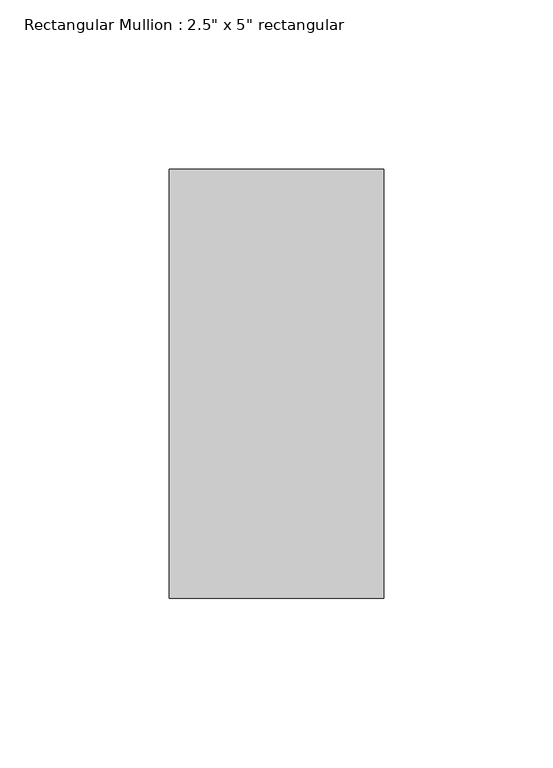
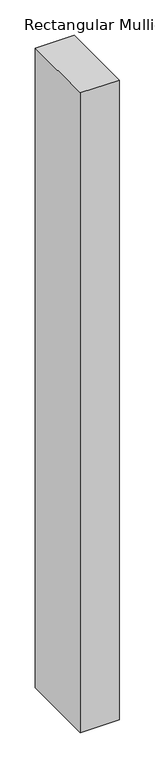
"""IFC4 building model written with IfcOpenShell, lengths in millimetres: member geometry."""

from ifc_helpers import new_model, si_unit, frame, origin, place, context, project, spatial, polyline, outline, extrude, source, transform, mapped, element, save


def member_88401a07(model_context):
    return source(origin(), model_context, "Body", "SweptSolid", [
        extrude(outline(polyline([(31.75, 63.5), (31.75, -63.5), (-31.75, -63.5), (-31.75, 63.5), (31.75, 63.5)])), frame((0.0, 0.0, -1102.7842439), z_axis=(0.0, 0.0, 1.0), x_axis=(1.0, 0.0, 0.0)), (0.0, 0.0, 1.0), 1102.7842439),
    ])


if __name__ == "__main__":
    model = new_model("IFC4")
    model_context = context("Model", 3, world=origin())
    ifc_project = project(units=[si_unit("LENGTHUNIT", "METRE", prefix="MILLI")], contexts=[model_context])
    site = spatial("IfcSite", under=ifc_project)
    building = spatial("IfcBuilding", under=site)
    placement = place(None, origin())
    member_shape = member_88401a07(model_context)
    element("IfcMember", 1, ObjectType="Rectangular Mullion : 2.5\" x 5\" rectangular", at=placement, inside=building, context=model_context, shape_type="MappedRepresentation", body=[
        mapped(member_shape, transform((0.0, 0.0, 0.0), x_axis=(1.0, 0.0, 0.0), y_axis=(0.0, 1.0, 0.0), z_axis=(0.0, 0.0, 1.0))),
    ])
    save(model, "model.ifc")

# Revit data of these elements
# Type "Rectangular Mullion : 2.5\" x 5\" rectangular"
#   built-in parameter 1007304 = 0.416667 (stored number, unit not read)
#   built-in parameter 1007301 = 0.104167 (stored number, unit not read)
#   built-in parameter 1007300 = 0.104167 (stored number, unit not read)
# Element 1 (IfcMember, "Rectangular Mullion : 2.5\" x 5\" rectangular")
#   Materials on its faces: "Aluminum"
# Materials
#   "Aluminum": class "Metal", colour RGB 247 247 247, transparency 0, Description = "Aluminum 6061", Cost = 0
